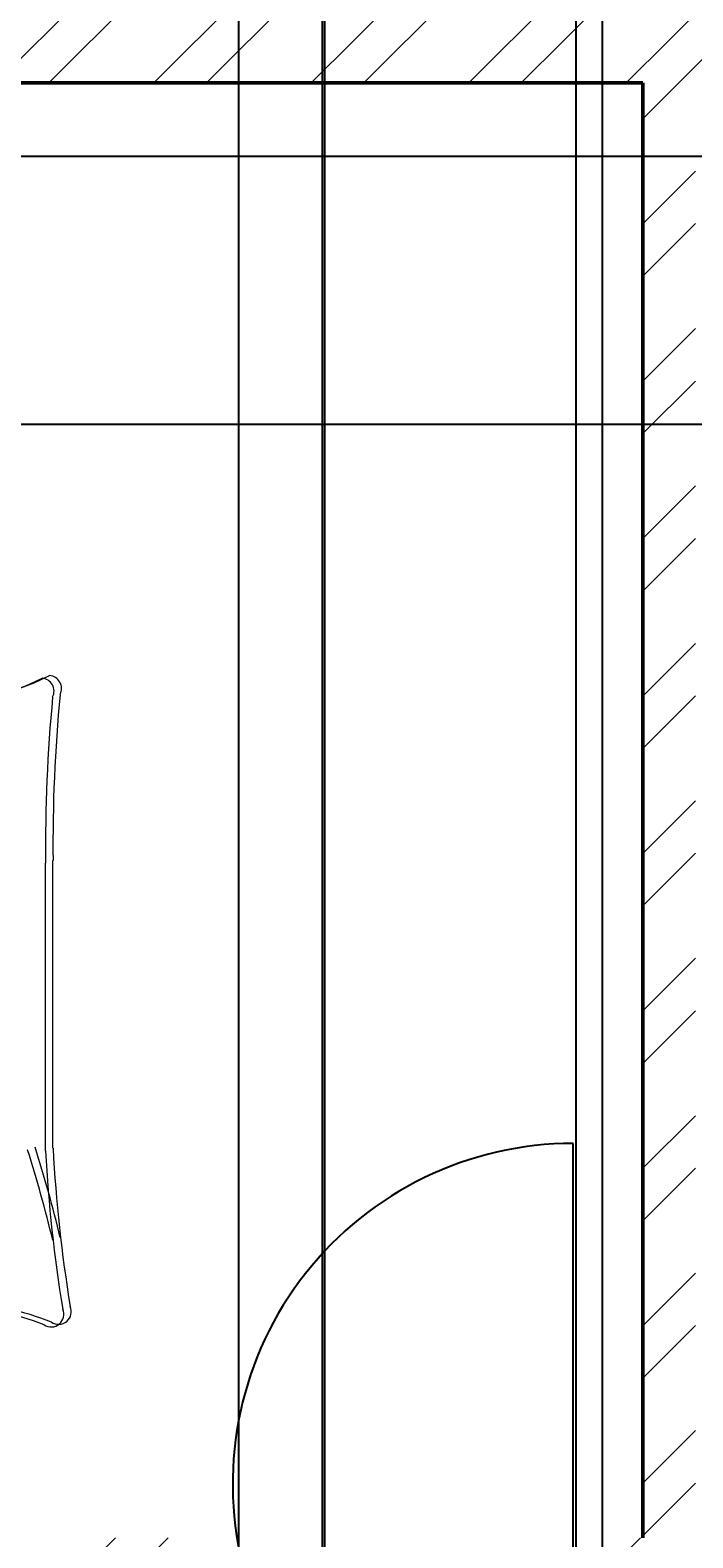
# Model space of a CAD drawing. Units: inches. Extents: x 1980 to 2738, y 1471 to 2568.
# Tile 8 of 22: x 2194 to 2250, y 1878 to 2007. Entities that reach past the tile are written whole.
import ezdxf

# ---------------------------------------------------------------- set-up
doc = ezdxf.new("R2010")
doc.units = ezdxf.units.IN
for name, color, linetype, lineweight in [('A-ANNO-DIMS', 2, 'Continuous', 18), ('A-DOOR', 31, 'Continuous', 25), ('A-FURN', 8, 'Continuous', 18), ('A-WALL', 7, 'Continuous', 50)]:
    doc.layers.add(name, color=color, linetype=linetype, lineweight=lineweight)
doc.layers.add('A-WALL-PATT', color=9, linetype='Continuous', lineweight=13, true_color=0xd19cc7)
doc.styles.get("Standard").update_dxf_attribs({"font": 'arial.ttf'})
doc.dimstyles.get("Standard").update_dxf_attribs({"dimtxt": 0.18, "dimasz": 0.18, "dimexe": 0.18, "dimexo": 0.0625, "dimgap": 0.09, "dimtad": 0, "dimtih": 1, "dimtoh": 1, "dimdec": 4, "dimzin": 0, "dimdsep": 46, "dimtxsty": 'Standard', "dimcen": 0.09, "dimadec": 0, "dimazin": 0, "dimtfac": 1, "dimtdec": 4, "dimtofl": 0, "dimtmove": 0, "dimatfit": 3, "dimfxl": 1, "dimtolj": 1, "dimtzin": 0, "dimarcsym": 0})

# ---------------------------------------------------------------- blocks, each defined once
blk = doc.blocks.new('BED-DOUBLE')
for p, q in [((28.38, 53.1), (25.13, 49.39)), ((28.38, 53.1), (25.13, 49.39)), ((29.49, 52.95), (27.75, 52.87, 3.87)), ((29.49, 52.95), (27.75, 52.87, 3.87)), ((30.13, 53.18), (28.38, 53.1, 3.87)), ((30.13, 53.18), (28.38, 53.1, 3.87)), ((29, 51.56), (28.38, 53.1)), ((29, 51.56), (28.38, 53.1)), ((27.75, 52.87), (24.5, 49.16)), ((27.75, 52.87), (24.5, 49.16)), ((28.36, 51.33), (27.75, 52.87)), ((28.36, 51.33), (27.75, 52.87)), ((0, 51.49), (0.64, 51.49)), ((0, 51.27), (26.61, 51.27)), ((0, 51.27), (26.61, 51.27)), ((0, 51.27), (0, 3.48)), ((0.64, 51.49), (27.25, 51.49)), ((0.64, 51.49), (27.25, 51.49)), ((1.53, 3.48), (1.53, 51.27)), ((1.53, 3.48), (1.53, 51.27)), ((2.17, 3.7), (2.17, 51.49)), ((2.17, 3.7), (2.17, 51.49)), ((3.2, 50.34), (3.1, 44.94)), ((3.2, 50.34), (3.1, 44.94)), ((3.2, 50.34), (6.41, 49.96)), ((3.2, 50.34), (6.41, 49.96)), ((5.77, 49.73), (8.34, 50.33)), ((5.77, 49.73), (8.34, 50.33)), ((6.41, 49.96), (8.98, 50.56)), ((6.41, 49.96), (8.98, 50.56)), ((8.34, 50.33), (9.38, 49.81)), ((8.34, 50.33), (9.38, 49.81)), ((12.47, 50.34), (8.9, 49.54)), ((12.47, 50.34), (8.9, 49.54)), ((8.98, 50.56), (10.02, 50.04)), ((8.98, 50.56), (10.02, 50.04)), ((14.07, 50.15), (12.47, 50.34)), ((14.07, 50.15), (12.47, 50.34)), ((16.57, 50.7), (13.43, 49.92)), ((16.57, 50.7), (13.43, 49.92)), ((17.21, 50.93), (14.07, 50.15)), ((17.21, 50.93), (14.07, 50.15)), ((16.17, 45.57), (16.57, 50.7)), ((16.17, 45.57), (16.57, 50.7)), ((16.81, 45.8), (17.21, 50.93)), ((16.81, 45.79), (17.21, 50.93)), ((28.06, 48.23), (28.36, 51.33)), ((28.06, 48.23), (28.36, 51.33)), ((28.69, 48.46), (29, 51.56)), ((28.69, 48.46), (29, 51.56)), ((2.56, 50.11), (2.46, 44.71)), ((2.56, 50.11), (2.46, 44.71)), ((2.56, 50.11), (5.77, 49.73)), ((2.56, 50.11), (5.77, 49.73)), ((8.26, 49.31), (5.58, 48.13)), ((8.26, 49.31), (5.58, 48.13)), ((8.9, 49.54), (6.22, 48.36)), ((8.9, 49.54), (6.22, 48.36)), ((11.83, 50.11), (8.26, 49.31)), ((11.83, 50.11), (8.26, 49.31)), ((13.43, 49.92), (11.83, 50.11)), ((13.43, 49.92), (11.83, 50.11)), ((24.5, 49.16), (22.33, 46.22)), ((24.5, 49.16), (22.33, 46.22)), ((25.13, 49.39), (22.97, 46.45)), ((25.13, 49.39), (22.97, 46.45)), ((28.36, 44.36), (28.06, 48.23)), ((28.36, 44.36), (28.06, 48.23)), ((29, 44.59), (28.69, 48.46)), ((29, 44.59), (28.69, 48.46)), ((22.97, 46.45), (20.96, 40.87)), ((22.97, 46.45), (20.96, 40.87)), ((2.46, 44.71), (2.54, 45.71)), ((2.46, 44.71), (2.54, 45.71)), ((2.54, 45.71), (3.07, 41.91)), ((2.54, 45.71), (3.07, 41.91)), ((3.1, 44.94), (3.18, 45.94)), ((3.1, 44.94), (3.18, 45.94)), ((3.18, 45.94), (3.71, 42.14)), ((3.18, 45.94), (3.71, 42.14)), ((16.73, 43.61), (16.17, 45.57)), ((16.73, 43.61), (16.17, 45.57)), ((17.37, 43.83), (16.81, 45.8)), ((17.37, 43.83), (16.81, 45.79)), ((22.33, 46.22), (20.32, 40.64)), ((22.33, 46.22), (20.32, 40.64)), ((28.83, 40.95), (28.36, 44.36)), ((28.83, 40.95), (28.36, 44.36)), ((29.47, 41.18), (29, 44.59)), ((29.47, 41.18), (29, 44.59)), ((16.29, 36.6), (16.73, 43.61)), ((16.29, 36.6), (16.73, 43.61)), ((16.93, 36.82), (17.37, 43.83)), ((16.93, 36.82), (17.37, 43.83)), ((3.07, 41.91), (4.42, 36.5)), ((3.07, 41.91), (4.42, 36.5)), ((3.71, 42.14), (5.06, 36.72)), ((3.71, 42.14), (5.06, 36.72)), ((20.32, 40.64), (17.38, 32.31)), ((20.32, 40.64), (17.38, 32.31)), ((20.96, 40.87), (18.02, 32.53)), ((20.96, 40.87), (18.02, 32.53)), ((29.76, 38.94), (28.83, 40.95)), ((29.76, 38.94), (28.83, 40.95)), ((30.4, 39.17), (29.47, 41.18)), ((30.4, 39.17), (29.47, 41.18)), ((3.67, 39.2), (3.08, 37.14)), ((3.67, 39.2), (3.08, 37.14)), ((4.31, 39.43), (3.72, 37.36)), ((4.31, 39.43), (3.72, 37.36)), ((30.38, 36.46), (29.76, 38.94)), ((30.38, 36.46), (29.76, 38.94)), ((31.02, 36.69), (30.4, 39.17)), ((31.02, 36.69), (30.4, 39.17)), ((79.24, 15.06), (79.24, 39.68)), ((79.24, 15.06), (79.24, 39.68)), ((79.88, 15.29), (79.88, 39.91)), ((79.88, 15.29), (79.88, 39.91)), ((3.08, 37.14), (2.54, 34.2)), ((3.08, 37.14), (2.54, 34.2)), ((3.72, 37.36), (3.18, 34.43)), ((3.72, 37.36), (3.18, 34.43)), ((15.63, 32.56), (16.29, 36.6)), ((15.63, 32.56), (16.29, 36.6)), ((16.27, 32.79), (16.93, 36.82)), ((16.27, 32.79), (16.93, 36.82)), ((23.88, 34.45), (28.36, 36.15)), ((23.88, 34.45), (28.36, 36.15)), ((24.52, 34.68), (29, 36.38)), ((24.52, 34.68), (29, 36.38)), ((28.36, 36.15), (30.38, 36.46)), ((28.36, 36.15), (30.38, 36.46)), ((29, 36.38), (31.02, 36.69)), ((29, 36.38), (31.02, 36.69)), ((2.54, 34.2), (2.56, 33.88)), ((2.54, 34.2), (2.56, 33.88)), ((2.56, 33.88), (2.98, 29.46)), ((2.56, 33.88), (2.98, 29.46)), ((3.18, 34.43), (3.2, 34.11)), ((3.18, 34.43), (3.2, 34.11)), ((3.2, 34.11), (3.62, 29.68)), ((3.2, 34.11), (3.62, 29.68)), ((16.74, 30.75), (15.45, 33.82)), ((16.74, 30.75), (15.45, 33.82)), ((17.38, 30.98), (16.09, 34.05)), ((17.38, 30.98), (16.09, 34.05)), ((17.38, 30.26), (23.88, 34.45)), ((17.38, 30.26), (23.88, 34.45)), ((18.02, 30.49), (24.52, 34.68)), ((18.02, 30.49), (24.52, 34.68)), ((17.53, 28.53), (17.38, 30.98)), ((17.53, 28.53), (17.38, 30.98)), ((3.62, 29.68), (3.13, 28.21)), ((3.62, 29.68), (3.13, 28.21)), ((16.89, 28.3), (16.74, 30.75)), ((16.89, 28.3), (16.74, 30.75)), ((2.98, 29.46), (2.49, 27.98)), ((2.98, 29.46), (2.49, 27.98)), ((14.86, 28.36), (17.53, 28.53)), ((14.86, 28.36), (17.53, 28.53)), ((2.49, 27.98), (7.87, 27.73)), ((2.49, 27.98), (7.87, 27.73)), ((3.13, 28.21), (8.51, 27.96)), ((3.13, 28.21), (8.51, 27.96)), ((7.22, 26.56), (10.4, 27.14)), ((7.22, 26.56), (10.4, 27.14)), ((7.86, 26.79), (11.04, 27.37)), ((7.86, 26.79), (11.04, 27.37)), ((7.87, 27.73), (11.08, 27.36)), ((7.87, 27.73), (11.08, 27.35)), ((8.51, 27.96), (11.72, 27.58)), ((8.51, 27.96), (11.72, 27.58)), ((10.4, 27.14), (11.7, 27.14)), ((10.4, 27.14), (11.7, 27.14)), ((11.04, 27.37), (12.34, 27.37)), ((11.04, 27.37), (12.34, 27.37)), ((11.08, 27.36), (12.38, 27.44)), ((11.08, 27.35), (12.38, 27.44)), ((11.7, 27.14), (13.58, 26.56)), ((11.7, 27.14), (13.58, 26.56)), ((11.72, 27.58), (13.02, 27.66)), ((11.72, 27.58), (13.02, 27.66)), ((12.34, 27.37), (14.22, 26.79)), ((12.34, 27.37), (14.22, 26.79)), ((12.38, 27.44), (14.22, 28.13)), ((12.38, 27.44), (14.22, 28.13)), ((13.02, 27.66), (14.86, 28.36)), ((13.02, 27.66), (14.86, 28.36)), ((14.22, 28.13), (16.89, 28.3)), ((14.22, 28.13), (16.89, 28.3)), ((1.87, 25.98), (7.22, 26.56)), ((1.87, 25.98), (7.22, 26.56)), ((2.45, 24.54), (1.87, 25.98)), ((2.45, 24.54), (1.87, 25.98)), ((2.51, 26.21), (7.86, 26.79)), ((2.51, 26.21), (7.86, 26.79)), ((3.09, 24.77), (2.51, 26.21)), ((3.09, 24.77), (2.51, 26.21)), ((13.58, 26.56), (16.26, 26.56)), ((13.58, 26.56), (16.26, 26.56)), ((14.22, 26.79), (16.9, 26.79)), ((14.22, 26.79), (16.9, 26.79)), ((16.26, 26.56), (16.26, 24.1)), ((16.26, 26.56), (16.26, 24.1)), ((16.9, 26.79), (16.9, 24.33)), ((16.9, 26.79), (16.9, 24.33)), ((2.3, 20.09), (2.45, 24.54)), ((2.3, 20.09), (2.45, 24.54)), ((2.94, 20.32), (3.09, 24.77)), ((2.94, 20.32), (3.09, 24.77)), ((16.17, 19.38), (16.57, 24.52)), ((16.17, 19.38), (16.57, 24.52)), ((16.81, 19.61), (17.21, 24.74)), ((16.81, 19.61), (17.21, 24.74)), ((16.26, 24.1), (15.17, 20.96)), ((16.26, 24.1), (15.17, 20.96)), ((16.9, 24.33), (15.81, 21.19)), ((16.9, 24.33), (15.81, 21.19)), ((2.3, 19.77), (2.3, 20.09)), ((2.3, 19.77), (2.3, 20.09)), ((3.03, 16.88), (2.3, 19.77)), ((3.03, 16.88), (2.3, 19.77)), ((2.94, 20), (2.94, 20.32)), ((2.94, 20), (2.94, 20.32)), ((3.67, 17.11), (2.94, 20)), ((3.67, 17.11), (2.94, 20)), ((16.73, 17.42), (16.17, 19.38)), ((16.73, 17.42), (16.17, 19.38)), ((17.37, 17.65), (16.81, 19.61)), ((17.37, 17.65), (16.81, 19.61)), ((3.75, 14.86), (3.03, 16.88)), ((3.75, 14.85), (3.03, 16.88)), ((3.32, 12.11), (4.33, 17.6)), ((3.32, 12.11), (4.33, 17.6)), ((4.39, 15.08), (3.67, 17.11)), ((4.39, 15.08), (3.67, 17.11)), ((3.96, 12.34), (4.97, 17.83)), ((3.96, 12.34), (4.97, 17.83)), ((16.29, 10.41), (16.73, 17.42)), ((16.29, 10.41), (16.73, 17.42)), ((16.93, 10.64), (17.37, 17.65)), ((16.93, 10.64), (17.37, 17.65)), ((3.03, 8.29), (3.32, 12.11)), ((3.03, 8.28), (3.32, 12.11)), ((3.67, 8.51), (3.96, 12.34)), ((3.67, 8.51), (3.96, 12.34)), ((15.63, 6.38), (16.29, 10.41)), ((15.63, 6.38), (16.29, 10.41)), ((16.27, 6.61), (16.93, 10.64)), ((16.27, 6.61), (16.93, 10.64)), ((16.29, 10.41), (16.62, 9.28)), ((16.29, 10.41), (16.62, 9.28)), ((16.93, 10.64), (17.26, 9.51)), ((16.93, 10.64), (17.26, 9.51)), ((16.62, 9.28), (17.34, 4.18)), ((16.62, 9.28), (17.34, 4.18)), ((17.26, 9.51), (17.98, 4.41)), ((17.26, 9.51), (17.98, 4.41)), ((3.01, 8.18), (3.03, 8.29)), ((3.01, 8.18), (3.03, 8.28)), ((3.34, 3.9), (3.01, 8.18)), ((3.34, 3.9), (3.01, 8.18)), ((3.65, 8.41), (3.67, 8.51)), ((3.65, 8.41), (3.67, 8.51)), ((3.98, 4.13), (3.65, 8.41)), ((3.98, 4.13), (3.65, 8.41)), ((8.95, 5.05), (6.21, 6.06)), ((8.95, 5.05), (6.21, 6.06)), ((9.59, 5.28), (6.85, 6.29)), ((9.59, 5.28), (6.85, 6.29)), ((13.21, 4.7), (9.59, 5.28)), ((13.21, 4.7), (9.59, 5.28)), ((3.32, 3.89), (6.5, 4.47)), ((3.32, 3.89), (6.5, 4.47)), ((3.96, 4.12), (7.14, 4.7)), ((3.96, 4.12), (7.14, 4.7)), ((6.5, 4.47), (9.1, 4.04)), ((6.5, 4.47), (9.1, 4.04)), ((7.14, 4.7), (9.74, 4.27)), ((7.14, 4.7), (9.74, 4.27)), ((12.57, 4.47), (8.95, 5.05)), ((12.57, 4.47), (8.95, 5.05)), ((9.1, 4.04), (10.11, 4.62)), ((9.1, 4.04), (10.11, 4.62)), ((9.74, 4.27), (10.75, 4.85)), ((9.74, 4.27), (10.75, 4.85)), ((14.16, 4.76), (12.57, 4.47)), ((14.16, 4.76), (12.57, 4.47)), ((14.8, 4.99), (13.21, 4.7)), ((14.8, 4.99), (13.21, 4.7)), ((17.34, 4.18), (14.16, 4.76)), ((17.34, 4.18), (14.16, 4.76)), ((17.98, 4.41), (14.8, 4.99)), ((17.98, 4.41), (14.8, 4.99)), ((18.11, 3.48), (0, 3.48)), ((18.11, 3.48), (0, 3.48)), ((18.75, 3.7), (0.64, 3.7)), ((18.75, 3.7), (0.64, 3.7))]:
    blk.add_line(p, q)
for centre, radius, start, end in [((68.67, 76.16), 23.07, 267.4714, 296.4681), ((68.67, 76.16), 23.07, 267.4714, 296.4681), ((69.31, 76.39), 23.07, 267.4714, 296.4681), ((69.31, 76.39), 23.07, 267.4714, 296.4681), ((78.87, 54.41), 1.1, 332.6588, 86.02), ((78.87, 54.41), 1.1, 332.6588, 86.02), ((79.51, 54.64), 1.1, 332.6588, 86.02), ((79.51, 54.64), 1.1, 332.6588, 86.02), ((-6.66, 51.33), 36.18, 349.8763, 2.5657), ((-6.66, 51.33), 36.18, 349.8763, 2.5657), ((36.31, 182.27), 129.5, 266.9791, 273.8365), ((36.31, 182.27), 129.5, 266.9791, 273.8365), ((-6.02, 51.56), 36.18, 349.8763, 2.5657), ((-6.02, 51.56), 36.18, 349.8763, 2.5657), ((36.95, 182.49), 129.5, 266.9791, 273.8365), ((36.95, 182.49), 129.5, 266.9791, 273.8365), ((67.82, -4508.74), 4561.86, 90.00217, 90.28689), ((67.82, -4508.74), 4561.86, 90.00217, 90.28689), ((68.46, -4508.51), 4561.86, 90.00217, 90.28689), ((68.46, -4508.52), 4561.86, 90.00217, 90.28689), ((212.28, 41.15), 133.04, 174.4998, 180.6351), ((212.28, 41.15), 133.04, 174.4998, 180.6351), ((212.92, 41.38), 133.04, 174.4998, 180.6351), ((212.92, 41.38), 133.04, 174.4998, 180.6351), ((35.71, 43.97), 6.22, 168.6608, 203.7384), ((35.71, 43.97), 6.22, 168.6608, 203.7384), ((35.07, 43.74), 6.22, 168.6608, 203.7384), ((35.07, 43.74), 6.22, 168.6608, 203.7384), ((2.12, 31.38), 29.65, 10.6617, 19.8806), ((2.12, 31.38), 29.65, 10.6617, 19.8806), ((1.48, 31.15), 29.65, 10.6617, 19.8806), ((1.48, 31.15), 29.65, 10.6617, 19.8806), ((156.32, 17.76), 129.02, 171.7845, 186.9006), ((156.32, 17.76), 129.02, 171.7845, 186.9006), ((156.96, 17.98), 129.02, 171.7845, 186.9006), ((156.96, 17.98), 129.02, 171.7845, 186.9006), ((30.44, 36.64), 0.185, 250.2464, 1.1377), ((30.44, 36.64), 0.185, 250.2464, 1.1377), ((31.08, 36.86), 0.185, 250.2464, 1.1377), ((31.08, 36.86), 0.185, 250.2464, 1.1377), ((182.05, 21.36), 164.97, 176.0865, 186.7821), ((182.05, 21.36), 164.97, 176.0865, 186.7821), ((182.69, 21.59), 164.97, 176.0865, 186.7821), ((182.69, 21.59), 164.97, 176.0865, 186.7821), ((-23.71, -17.22), 106.46, 13.3832, 17.7053), ((-23.71, -17.22), 106.46, 13.3832, 17.7053), ((-23.07, -16.99), 106.46, 13.3832, 17.7053), ((-23.07, -16.99), 106.46, 13.3832, 17.7053), ((200.84, 21.43), 121.76, 182.9958, 189.4091), ((200.84, 21.43), 121.76, 182.9958, 189.4091), ((201.48, 21.66), 121.76, 182.9958, 189.4091), ((201.48, 21.66), 121.76, 182.9958, 189.4091), ((31.17, -167.31), 170.11, 88.4762, 91.0082), ((31.17, -167.31), 170.11, 88.4762, 91.0082), ((31.81, -167.08), 170.11, 88.4762, 91.0082), ((31.81, -167.08), 170.11, 88.4762, 91.0082), ((50.61, 484.82), 482.31, 268.2277, 271.7185), ((50.61, 484.82), 482.31, 268.2277, 271.7185), ((51.25, 485.05), 482.31, 268.2277, 271.7185), ((51.25, 485.05), 482.31, 268.2277, 271.7185), ((64.51, -26.9), 29.63, 76.0648, 88.9113), ((64.51, -26.9), 29.63, 76.0648, 88.9113), ((65.15, -26.67), 29.63, 76.0648, 88.9113), ((65.15, -26.67), 29.63, 76.0648, 88.9113), ((20.1, 85.16), 83.31, 268.7218, 275.604), ((20.1, 85.16), 83.31, 268.7218, 275.604), ((20.74, 85.39), 83.31, 268.7218, 275.604), ((20.74, 85.39), 83.31, 268.7218, 275.604), ((70.28, -21.66), 23.56, 67.9751, 86.652), ((70.28, -21.66), 23.56, 67.9751, 86.652), ((70.91, -21.43), 23.56, 67.9751, 86.652), ((70.91, -21.43), 23.56, 67.9751, 86.652), ((79.72, 1.09), 1.09, 236.1736, 23.4781), ((79.72, 1.09), 1.09, 236.1736, 23.4781), ((80.36, 1.32), 1.09, 236.1736, 23.4781), ((80.36, 1.32), 1.09, 236.1736, 23.4781)]:
    blk.add_arc(centre, radius, start, end)
blk = doc.blocks.new('*D40')
at = {"layer": 'A-ANNO-DIMS', "color": 0, "lineweight": -2, "transparency": 16777216}
for p, q in [((2218.65, 2053.14), (2218.65, 1533.71)), ((2298.65, 2053.14), (2298.65, 1533.71)), ((2218.83, 1533.89), (2258.43, 1533.89)), ((2298.47, 1533.89), (2258.87, 1533.89))]:
    blk.add_line(p, q, dxfattribs=at)
at = {"layer": 'A-ANNO-DIMS', "color": 0, "transparency": 16777216}
for points in [[(2218.83, 1533.92), (2218.83, 1533.86), (2218.65, 1533.89)], [(2298.47, 1533.92), (2298.47, 1533.86), (2298.65, 1533.89)]]:
    blk.add_solid(points, dxfattribs=at)
at = {"layer": 'Defpoints', "color": 0, "transparency": 16777216}
for p in [(2218.65, 2053.21), (2298.65, 2053.21), (2298.65, 1533.89)]:
    blk.add_point(p, dxfattribs=at)
at = {"layer": 'A-ANNO-DIMS', "color": 0, "transparency": 16777216, "insert": (2258.65, 1533.89), "char_height": 0.18, "attachment_point": 5}
blk.add_mtext('\\A1;80', dxfattribs=at)
blk = doc.blocks.new('*D44')
at = {"layer": 'A-ANNO-DIMS', "color": 0, "lineweight": -2, "transparency": 16777216}
for p, q in [((2218.88, 1694.77), (2218.88, 2507.54)), ((2219.06, 2507.36), (2229.18, 2507.36)), ((2240.22, 2507.36), (2230.11, 2507.36)), ((2240.4, 1694.77), (2240.4, 2507.54))]:
    blk.add_line(p, q, dxfattribs=at)
at = {"layer": 'A-ANNO-DIMS', "color": 0, "transparency": 16777216}
for points in [[(2219.06, 2507.39), (2219.06, 2507.33), (2218.88, 2507.36)], [(2240.22, 2507.39), (2240.22, 2507.33), (2240.4, 2507.36)]]:
    blk.add_solid(points, dxfattribs=at)
at = {"layer": 'Defpoints', "color": 0, "transparency": 16777216}
for p in [(2240.4, 2507.36), (2218.88, 1694.71), (2240.4, 1694.71)]:
    blk.add_point(p, dxfattribs=at)
at = {"layer": 'A-ANNO-DIMS', "color": 0, "transparency": 16777216, "insert": (2229.64, 2507.36), "char_height": 0.18, "attachment_point": 5}
blk.add_mtext('\\A1;21.525', dxfattribs=at)
blk = doc.blocks.new('*D46')
at = {"layer": 'A-ANNO-DIMS', "color": 0, "lineweight": -2, "transparency": 16777216}
for p, q in [((2211.52, 1814.77), (2211.52, 2507.54)), ((2211.7, 2507.36), (2226.69, 2507.36)), ((2242.46, 2507.36), (2227.48, 2507.36)), ((2242.64, 1814.77), (2242.64, 2507.54))]:
    blk.add_line(p, q, dxfattribs=at)
at = {"layer": 'A-ANNO-DIMS', "color": 0, "transparency": 16777216}
for points in [[(2211.7, 2507.39), (2211.7, 2507.33), (2211.52, 2507.36)], [(2242.46, 2507.39), (2242.46, 2507.33), (2242.64, 2507.36)]]:
    blk.add_solid(points, dxfattribs=at)
at = {"layer": 'Defpoints', "color": 0, "transparency": 16777216}
for p in [(2242.64, 2507.36), (2211.52, 1814.71), (2242.64, 1814.71)]:
    blk.add_point(p, dxfattribs=at)
at = {"layer": 'A-ANNO-DIMS', "color": 0, "transparency": 16777216, "insert": (2227.08, 2507.36), "char_height": 0.18, "attachment_point": 5}
blk.add_mtext('\\A1;31.12', dxfattribs=at)
blk = doc.blocks.new('*D56')
at = {"layer": 'A-ANNO-DIMS', "color": 0, "lineweight": -2, "transparency": 16777216}
for p, q in [((2114.15, 1995.93), (2689.91, 1995.93)), ((2689.73, 1995.75), (2689.73, 1984.65)), ((2689.73, 1973.18), (2689.73, 1984.28)), ((2114.15, 1973), (2689.91, 1973))]:
    blk.add_line(p, q, dxfattribs=at)
at = {"layer": 'A-ANNO-DIMS', "color": 0, "transparency": 16777216}
for points in [[(2689.7, 1995.75), (2689.76, 1995.75), (2689.73, 1995.93)], [(2689.7, 1973.18), (2689.76, 1973.18), (2689.73, 1973)]]:
    blk.add_solid(points, dxfattribs=at)
at = {"layer": 'Defpoints', "color": 0, "transparency": 16777216}
for p in [(2114.08, 1995.93), (2689.73, 1995.93), (2114.08, 1973)]:
    blk.add_point(p, dxfattribs=at)
at = {"layer": 'A-ANNO-DIMS', "color": 0, "transparency": 16777216, "insert": (2689.73, 1984.47), "char_height": 0.18, "attachment_point": 5}
blk.add_mtext('\\A1;22.935', dxfattribs=at)

msp = doc.modelspace()

# ---------------------------------------------------------------- hatches: boundary and pattern name
at = {"layer": 'A-WALL-PATT'}
h = msp.add_hatch(dxfattribs=at)
h.set_pattern_fill('ANSI32', color=256)
h.paths.add_polyline_path([(2257.5661, 2416.2064), (2257.5661, 2420.7064), (2250.5833, 2420.7064), (2250.5833, 2462.7064), (2246.0833, 2462.7064), (2246.0833, 2420.7064), (2237.0791, 2420.7064), (2237.0791, 2411.7064), (2246.0833, 2411.7064), (2246.0833, 2291.7064), (2242.6109, 2291.7064), (2242.6109, 2287.2064), (2246.0833, 2287.2064), (2250.5833, 2287.2064), (2250.5833, 2291.7064), (2250.5833, 2411.7064), (2257.5661, 2411.7064)])
h.paths.add_polyline_path([(2387.0396, 2416.2064), (2387.0396, 2420.7064), (2367.5833, 2420.7064), (2367.5833, 2462.7064), (2358.5833, 2462.7064), (2358.5833, 2420.7064), (2329.3087, 2420.7064), (2329.3087, 2411.7064), (2358.5833, 2411.7064), (2358.5833, 2321.7275), (2358.5833, 2309.7064), (2347.3089, 2309.7064), (2293.3089, 2309.7064), (2293.3089, 2259.0771), (2297.8089, 2259.0771), (2297.8089, 2305.2064), (2347.3089, 2305.2064), (2347.3089, 2284.7412), (2351.8089, 2284.7412), (2351.8089, 2305.2064), (2372.3188, 2305.2064), (2372.3761, 2284.3899), (2377.0295, 2284.3899), (2377.0295, 2299.3058), (2377.0295, 2305.2064), (2426.5295, 2305.2064), (2426.5295, 2257.5573), (2431.0295, 2257.5573), (2431.0295, 2309.7064), (2377.0295, 2309.7064), (2367.5833, 2309.7064), (2367.5833, 2321.7275), (2367.5833, 2411.7064), (2387.0396, 2411.7064)])
h.paths.add_polyline_path([(2448.5267, 2416.2064), (2448.5267, 2420.7064), (2423.0396, 2420.7064), (2423.0396, 2411.7064), (2448.5267, 2411.7064)])
h.paths.add_polyline_path([(2130.9128, 2416.2064), (2130.9128, 2420.7064), (2105.0833, 2420.7064), (2105.0833, 2386.6942), (2114.0833, 2386.6942), (2114.0833, 2411.7064), (2130.9128, 2411.7064)])
h.paths.add_polyline_path([(2212.9478, 2420.7064), (2190.9128, 2420.7064), (2190.9128, 2411.7064), (2212.9478, 2411.7064), (2212.9478, 2416.2064)])
h.paths.add_polyline_path([(2114.0833, 2326.6942), (2105.0833, 2326.6942), (2105.0833, 2291.7064), (2081.0833, 2291.7064), (2081.0833, 2287.2064), (2105.0833, 2287.2064), (2105.0833, 2276.1935), (2114.0833, 2276.1935), (2114.0833, 2287.2064), (2166.3825, 2287.2064), (2166.3825, 2289.4564), (2166.3825, 2291.7064), (2114.0833, 2291.7064)])
h.paths.add_polyline_path([(2114.0833, 2252.1935), (2105.0833, 2252.1935), (2105.0833, 2233.2064), (2081.0833, 2233.2064), (2081.0833, 2228.7064), (2105.0833, 2228.7064), (2105.0833, 2213.4478), (2114.0833, 2213.4478), (2114.0833, 2228.7064), (2195.0833, 2228.7064), (2199.5833, 2228.7064), (2208.4455, 2228.7064), (2208.4455, 2230.9564), (2208.4455, 2233.2064), (2199.5833, 2233.2064), (2199.5833, 2287.2064), (2206.8904, 2287.2064), (2206.8904, 2289.4564), (2206.8904, 2291.7064), (2189.446, 2291.7064), (2189.446, 2289.4564), (2189.446, 2287.2064), (2195.0833, 2287.2064), (2195.0833, 2233.2064), (2114.0833, 2233.2064)])
h.paths.add_polyline_path([(2114.0833, 2153.4478), (2109.5833, 2153.4478), (2105.0833, 2153.4478), (2105.0833, 2135.2374), (2114.0833, 2135.2374)], flags=17)
h.paths.add_polyline_path([(2135.9619, 2095.4081), (2140.1805, 2095.4081), (2140.1805, 2104.2064), (2114.0833, 2104.2064), (2114.0833, 2110.3997), (2109.5833, 2110.3997), (2105.0833, 2110.3997), (2105.0833, 2104.2064), (2081.0833, 2104.2064), (2081.0833, 2099.7064), (2105.0833, 2099.7064), (2127.5416, 2099.8532), (2127.5416, 2056.9393), (2136.2133, 2056.9393)], flags=17)
h.paths.add_polyline_path([(2255.4895, 2104.2064), (2250.5833, 2104.2064), (2250.5833, 2233.2064), (2246.0833, 2233.2064), (2242.4941, 2233.2064), (2242.4941, 2228.7064), (2246.0833, 2228.7064), (2246.0833, 2104.2064), (2163.6825, 2104.2064), (2163.6825, 2099.8072), (2163.6825, 2095.4081), (2191.4325, 2095.4081), (2191.4325, 2011.2064), (2186.0833, 2011.2064), (2136.5143, 2010.8824), (2136.3702, 2032.9403), (2131.9559, 2032.9115), (2127.5416, 2032.8826), (2127.5416, 2006.7064), (2105.0833, 2006.7064), (2081.0833, 2006.7064), (2081.0833, 2002.2064), (2105.0833, 2002.2064), (2105.0833, 1995.9329), (2114.0833, 1995.9329), (2114.0833, 2002.2064), (2246.0833, 2002.2064), (2246.0833, 1877.7064), (2242.1358, 1877.7064), (2242.1358, 1873.2064), (2250.5833, 1873.2064), (2250.5833, 2002.2064), (2255.3335, 2002.2064), (2255.3335, 2011.2064), (2195.9325, 2011.2064), (2195.9325, 2095.2064), (2255.4895, 2095.2064), (2255.4895, 2099.5471)])
h.paths.add_polyline_path([(2199.5833, 1873.2064), (2209.827, 1873.2064), (2209.827, 1875.4564), (2209.827, 1877.7064), (2114.0833, 1877.7064), (2114.0833, 1890.0968), (2105.0833, 1890.0968), (2105.0833, 1877.7064), (2081.0833, 1877.7064), (2081.0833, 1873.2064), (2105.0833, 1873.2064), (2105.0833, 1857.7279), (2114.0833, 1857.7279), (2114.0833, 1873.2064), (2195.0833, 1873.2064), (2195.0833, 1819.2064), (2190.298, 1819.2064), (2190.298, 1814.7064), (2209.8976, 1814.7064), (2209.8976, 1816.9564), (2209.8976, 1819.2064), (2199.5833, 1819.2064)])
h.paths.add_polyline_path([(2114.0833, 1814.7064), (2166.2538, 1814.7064), (2166.2538, 1816.9564), (2166.2538, 1819.2064), (2114.0833, 1819.2064), (2114.0833, 1833.7279), (2109.5833, 1833.7279), (2105.0833, 1833.7279), (2105.0833, 1819.2064), (2081.0833, 1819.2064), (2081.0833, 1814.7064), (2105.0833, 1814.7064), (2105.0833, 1782.5516), (2114.0833, 1782.5516)])
h.paths.add_polyline_path([(2114.0833, 1722.5516), (2109.5833, 1722.5516), (2105.0833, 1722.5516), (2105.0833, 1685.7064), (2124.5104, 1685.7064), (2124.5104, 1690.2064), (2124.5104, 1694.7064), (2114.0833, 1694.7064)])
h.paths.add_polyline_path([(2218.8787, 1694.7064), (2184.5104, 1694.7064), (2184.5104, 1685.7064), (2218.8787, 1685.7064), (2218.8787, 1690.2064)])
h.paths.add_polyline_path([(2250.5833, 1819.2064), (2242.6431, 1819.2064), (2242.6431, 1816.9564), (2242.6431, 1814.7064), (2246.0833, 1814.7064), (2246.0833, 1694.7064), (2240.4035, 1694.7064), (2240.4035, 1690.2064), (2240.4035, 1685.7064), (2246.0833, 1685.7064), (2246.0833, 1643.7064), (2250.5833, 1643.7064), (2250.5833, 1685.7064), (2255.9859, 1685.7064), (2255.9859, 1690.2064), (2255.9859, 1694.7064), (2250.5833, 1694.7064)])
h.paths.add_polyline_path([(2297.4764, 1694.7064), (2279.3934, 1694.7064), (2279.3934, 1690.2064), (2279.3934, 1685.7064), (2297.4764, 1685.7064), (2297.4764, 1690.2064)])
h.paths.add_polyline_path([(2377.1596, 1694.7064), (2367.5833, 1694.7064), (2367.5833, 1787.7064), (2431.0295, 1787.7064), (2431.0295, 1792.2064), (2431.0295, 1849.4149), (2428.7795, 1849.4149), (2426.5295, 1849.4149), (2426.5295, 1792.2064), (2421.5833, 1792.2064), (2367.5833, 1792.2064), (2297.8089, 1792.2064), (2297.8089, 1850.2946), (2295.5589, 1850.2946), (2293.3089, 1850.2946), (2293.3089, 1792.2064), (2293.3089, 1787.7064), (2297.8089, 1787.7064), (2358.5833, 1787.7064), (2358.5833, 1694.7064), (2333.4764, 1694.7064), (2333.4764, 1685.7064), (2358.5833, 1685.7064), (2358.5833, 1643.7064), (2367.5833, 1643.7064), (2367.5833, 1685.7064), (2377.1596, 1685.7064)])
h.paths.add_polyline_path([(2442.4912, 1694.7064), (2413.1596, 1694.7064), (2413.1596, 1685.7064), (2442.4912, 1685.7064)])
h.paths.add_polyline_path([(2480.0833, 1814.7064), (2483.4816, 1814.7064), (2483.4816, 1817.9384), (2483.4816, 1819.2064), (2475.5833, 1819.2064), (2475.5833, 1694.7064), (2470.7283, 1694.7064), (2470.7283, 1685.7064), (2475.5833, 1685.7064), (2475.5833, 1643.7064), (2480.0833, 1643.7064), (2480.0833, 1685.7064), (2486.3293, 1685.7064), (2486.3293, 1690.2064), (2486.3293, 1694.7064), (2480.0833, 1694.7064)])
h.paths.add_polyline_path([(2621.0833, 1721.7349), (2612.0833, 1721.7349), (2612.0833, 1694.7064), (2586.1453, 1694.7064), (2586.1453, 1685.7064), (2621.0833, 1685.7064)])
h.paths.add_polyline_path([(2526.1453, 1690.2064), (2526.1453, 1694.7064), (2511.584, 1694.7064), (2511.584, 1690.2064), (2511.584, 1685.7064), (2526.1453, 1685.7064)])
h.paths.add_polyline_path([(2645.0833, 1819.2064), (2621.0833, 1819.2064), (2621.0833, 1835.8527), (2616.5833, 1835.8527), (2612.0833, 1835.8527), (2612.0833, 1819.2064), (2560.2541, 1819.2064), (2560.2541, 1814.7064), (2612.0833, 1814.7064), (2612.0833, 1781.7349), (2621.0833, 1781.7349), (2621.0833, 1814.7064), (2645.0833, 1814.7064)])
h.paths.add_polyline_path([(2645.0833, 1877.7064), (2621.0833, 1877.7064), (2621.0833, 1886.4375), (2612.0833, 1886.4375), (2612.0833, 1877.7064), (2517.1032, 1877.7064), (2517.1032, 1875.4564), (2517.1032, 1873.2064), (2526.5833, 1873.2064), (2526.5833, 1819.2064), (2516.6454, 1819.2064), (2516.6454, 1816.9564), (2516.6454, 1814.7064), (2536.4445, 1814.7064), (2536.4445, 1816.9564), (2536.4445, 1819.2064), (2531.0833, 1819.2064), (2531.0833, 1873.2064), (2612.0833, 1873.2064), (2612.0833, 1859.8527), (2621.0833, 1859.8527), (2621.0833, 1873.2064), (2645.0833, 1873.2064)])
h.paths.add_polyline_path([(2645.0833, 2006.7064), (2621.0833, 2006.7064), (2588.5085, 2006.7064), (2588.5085, 2052.9125), (2579.9045, 2052.9125), (2579.9045, 2011.2064), (2519.9045, 2011.2064), (2519.9045, 2095.2064), (2553.1204, 2095.2064), (2553.1204, 2104.2064), (2480.0833, 2104.2064), (2480.0833, 2228.7064), (2484.3832, 2228.7064), (2484.3832, 2230.9564), (2484.3832, 2233.2064), (2475.5833, 2233.2064), (2475.5833, 2104.2064), (2463.1308, 2104.2064), (2463.1308, 2095.2064), (2501.2463, 2095.2064), (2510.9045, 2095.2064), (2515.4045, 2095.2064), (2515.4045, 2011.2064), (2510.9045, 2011.2064), (2501.2463, 2011.2064), (2462.5957, 2011.2064), (2462.5957, 2002.2064), (2475.5833, 2002.2064), (2475.5833, 1873.2064), (2483.6146, 1873.2064), (2483.6146, 1875.4564), (2483.6146, 1877.7064), (2480.0833, 1877.7064), (2480.0833, 2002.2064), (2612.0833, 2002.2064), (2612.0833, 1996.309), (2621.0833, 1996.309), (2621.0833, 2002.2064), (2645.0833, 2002.2064)])
h.paths.add_polyline_path([(2588.5085, 2099.7277), (2621.0833, 2099.7277), (2645.0833, 2099.7064), (2645.0833, 2104.2064), (2621.0833, 2104.2064), (2621.0833, 2109.0038), (2616.5833, 2109.0038), (2612.0833, 2109.0038), (2612.0833, 2104.2064), (2575.0621, 2104.2064), (2575.0621, 2099.7064), (2575.0621, 2095.2064), (2579.9045, 2095.2064), (2579.9045, 2076.9125), (2588.5085, 2076.9125)], flags=17)
h.paths.add_polyline_path([(2367.5833, 2002.2064), (2373.7228, 2002.2064), (2373.7228, 2006.7064), (2373.7228, 2011.2064), (2350.7889, 2011.2064), (2350.7889, 2006.7064), (2350.7889, 2002.2064), (2358.5833, 2002.2064), (2358.5833, 1877.7064), (2293.3089, 1877.7064), (2293.3089, 1870.4987), (2297.8089, 1870.4987), (2297.8089, 1873.2064), (2347.3089, 1873.2064), (2347.3089, 1847.2208), (2351.8089, 1847.2208), (2351.8089, 1873.2064), (2372.5295, 1873.2064), (2372.5295, 1847.8619), (2377.0295, 1847.8619), (2377.0295, 1873.2064), (2426.5295, 1873.2064), (2426.5295, 1868.7339), (2431.0295, 1868.7339), (2431.0295, 1877.7064), (2367.5833, 1877.7064)])
h.paths.add_polyline_path([(2531.0833, 2287.2064), (2534.2285, 2287.2064), (2534.2285, 2291.7064), (2516.7886, 2291.7064), (2516.7886, 2287.2064), (2526.5833, 2287.2064), (2526.5833, 2233.2064), (2517.9112, 2233.2064), (2517.9112, 2230.9564), (2517.9112, 2228.7064), (2526.5833, 2228.7064), (2531.0833, 2228.7064), (2612.0833, 2228.7064), (2612.0833, 2206.8504), (2621.0833, 2206.8504), (2621.0833, 2228.7064), (2645.0833, 2228.7064), (2645.0833, 2233.2064), (2621.0833, 2233.2064), (2621.0833, 2241.8536), (2616.5833, 2241.8536), (2612.0833, 2241.8536), (2612.0833, 2233.2064), (2531.0833, 2233.2064)])
h.paths.add_polyline_path([(2645.0833, 2291.7064), (2621.0833, 2291.7064), (2621.0833, 2323.0138), (2616.5833, 2323.0138), (2612.0833, 2323.0138), (2612.0833, 2291.7064), (2559.6852, 2291.7064), (2559.6852, 2289.4564), (2559.6852, 2287.2064), (2612.0833, 2287.2064), (2612.0833, 2265.8536), (2621.0833, 2265.8536), (2621.0833, 2287.2064), (2645.0833, 2287.2064)])
h.paths.add_polyline_path([(2621.0833, 2420.7064), (2582.8189, 2420.7064), (2582.8189, 2411.7064), (2612.0833, 2411.7064), (2612.0833, 2383.0138), (2621.0833, 2383.0138)])
h.paths.add_polyline_path([(2480.0833, 2411.7064), (2485.7342, 2411.7064), (2485.7342, 2416.2064), (2485.7342, 2420.7064), (2480.0833, 2420.7064), (2480.0833, 2462.7064), (2475.5833, 2462.7064), (2475.5833, 2420.7064), (2469.4083, 2420.7064), (2469.4083, 2411.7064), (2475.5833, 2411.7064), (2475.5833, 2291.7064), (2475.5833, 2287.2064), (2482.9195, 2287.2064), (2482.9195, 2289.4564), (2482.9195, 2291.7064), (2480.0833, 2291.7064)])
h.paths.add_polyline_path([(2367.5833, 2228.7064), (2431.0295, 2228.7064), (2431.0295, 2233.2064), (2431.0295, 2237.4203), (2428.7795, 2237.4203), (2426.5295, 2237.4203), (2426.5295, 2233.2064), (2377.0295, 2233.2064), (2377.0295, 2260.3837), (2372.4423, 2260.3837), (2372.517, 2233.2635), (2351.8089, 2233.2064), (2351.8089, 2260.7412), (2347.3089, 2260.7412), (2347.3089, 2233.2064), (2297.8089, 2233.2064), (2297.8089, 2236.9324), (2293.3089, 2236.9324), (2293.3089, 2228.7064), (2358.5833, 2228.7064), (2358.5833, 2104.2064), (2353.3665, 2104.2064), (2353.3665, 2095.2064), (2373.8869, 2095.2064), (2373.8869, 2099.7064), (2373.8869, 2104.2064), (2367.5833, 2104.2064)])
h.paths.add_polyline_path([(2321.2323, 2104.2064), (2303.4895, 2104.2064), (2303.4895, 2095.2064), (2321.2323, 2095.2064), (2321.2323, 2099.7064)], flags=0)
h.paths.add_polyline_path([(2415.1308, 2099.7064), (2415.1308, 2104.2064), (2404.81, 2104.2064), (2404.81, 2095.2064), (2415.1308, 2095.2064)], flags=17)
h.paths.add_polyline_path([(2318.6336, 2011.2064), (2303.3335, 2011.2064), (2303.3335, 2002.2064), (2318.6336, 2002.2064)], flags=0)
h.paths.add_polyline_path([(2414.5957, 2011.2064), (2406.2461, 2011.2064), (2406.2461, 2006.7064), (2406.2461, 2002.2064), (2414.5957, 2002.2064)], flags=17)

# ---------------------------------------------------------------- linework, layer by layer
at = {"layer": 'A-DOOR'}
msp.add_line((2240.1358, 1875.4564), (2240.1358, 1911.4564), dxfattribs=at)
msp.add_arc((2240.1358, 1882.3261), 29.1304, 90, 193.640185, dxfattribs=at)
at = {"layer": 'A-WALL'}
for q in [(2114.0833, 2002.2064), (2246.0833, 1877.7064)]:
    msp.add_line((2246.0833, 2002.2064), q, dxfattribs=at)

# ---------------------------------------------------------------- block references
at = {"layer": 'A-FURN'}
msp.add_blockref('BED-DOUBLE', (2115.753, 1895.7455), dxfattribs=at)

# ---------------------------------------------------------------- dimensions: what is measured, and where the dimension line sits
at = {"layer": 'A-ANNO-DIMS'}
for base, p1, p2, override, picture, middle in [((2242.6431, 2507.3564), (2211.5238, 1814.7064), (2242.6431, 1814.7064), {"dimdec": 2, "dimlfac": 1, "dimrnd": 0, "dimzin": 0, "dimdsep": 46, "dimlunit": 2}, '*D46', (2227.0835, 2507.3564)), ((2240.4035, 2507.3564), (2218.8787, 1694.7064), (2240.4035, 1694.7064), {"dimdec": 3, "dimlfac": 1, "dimrnd": 0, "dimzin": 0, "dimdsep": 46, "dimlunit": 2}, '*D44', (2229.6411, 2507.3564)), ((2298.6516, 1533.8857), (2218.6516, 2053.2064), (2298.6516, 2053.2064), {"dimdec": 0, "dimlfac": 1, "dimrnd": 0, "dimzin": 0, "dimdsep": 46, "dimlunit": 2}, '*D40', (2258.6516, 1533.8857))]:
    dim = msp.add_linear_dim(base=base, p1=p1, p2=p2, dimstyle='Standard', override=override, dxfattribs=at)
    dim.commit()
    dim.dimension.update_dxf_attribs({"geometry": picture, "text_midpoint": middle})
dim = msp.add_linear_dim(base=(2689.7333, 1995.9329), p1=(2114.0833, 1972.9983), p2=(2114.0833, 1995.9329), angle=90, dimstyle='Standard', override={"dimdec": 3, "dimlfac": 1, "dimrnd": 0, "dimzin": 0, "dimdsep": 46, "dimlunit": 2}, dxfattribs=at)
dim.commit()
dim.dimension.update_dxf_attribs({"geometry": '*D56', "text_midpoint": (2689.7333, 1984.4656)})

doc.saveas('drawing.dxf')
